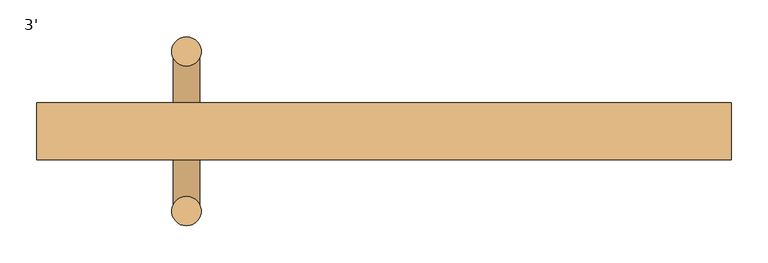
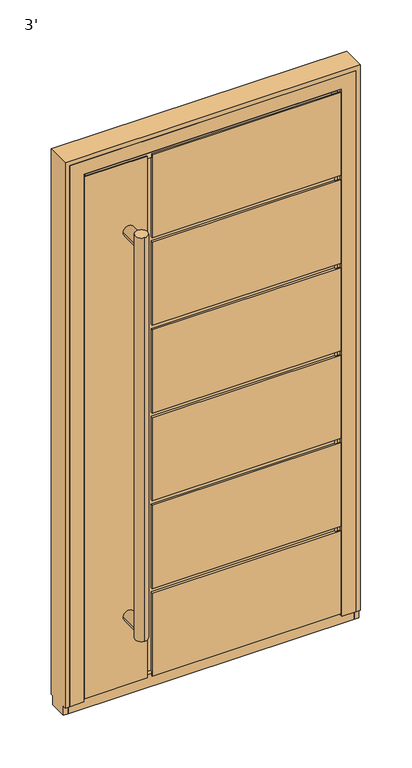
"""IFC4 building model written with IfcOpenShell, lengths in millimetres: door geometry, 3'."""

from ifc_helpers import new_model, si_unit, point, frame, frame_2d, origin, place, context, project, spatial, circle_curve, trimmed, segment, composite_curve, outline, extrude, faceted_brep, source, transform, mapped, element, save


def door_3_44036f4b(model_context):
    return source(origin(), model_context, "Body", "SolidModel", [
        extrude(outline(composite_curve([segment(trimmed(circle_curve(frame_2d((-268.65, 90.8003001)), 20.0), [point((-268.65, 70.8003001))], [point((-268.65, 110.8003001))], False, "CARTESIAN"), True, "CONTINUOUS"), segment(trimmed(circle_curve(frame_2d((-268.65, 90.8003001)), 20.0), [point((-268.65, 110.8003001))], [point((-268.65, 70.8003001))], False, "CARTESIAN"), True, "CONTINUOUS")], self_intersect=False)), frame((0.0, 0.0, 210.0000003), z_axis=(0.0, 0.0, 1.0), x_axis=(1.0, 0.0, 0.0)), (0.0, 0.0, 1.0), 1363.8),
        extrude(outline(composite_curve([segment(trimmed(circle_curve(frame_2d((-268.65, -126.2003001)), 20.0), [point((-268.65, -146.2003001))], [point((-268.65, -106.2003001))], False, "CARTESIAN"), True, "CONTINUOUS"), segment(trimmed(circle_curve(frame_2d((-268.65, -126.2003001)), 20.0), [point((-268.65, -106.2003001))], [point((-268.65, -146.2003001))], False, "CARTESIAN"), True, "CONTINUOUS")], self_intersect=False)), frame((0.0, 0.0, 210.0000003), z_axis=(0.0, 0.0, 1.0), x_axis=(1.0, 0.0, 0.0)), (0.0, 0.0, 1.0), 1363.8),
        extrude(outline(composite_curve([segment(trimmed(circle_curve(frame_2d((241.9000003, -268.65)), 18.0), [point((241.9000003, -286.65))], [point((241.9000003, -250.65))], False, "CARTESIAN"), True, "CONTINUOUS"), segment(trimmed(circle_curve(frame_2d((241.9000003, -268.65)), 18.0), [point((241.9000003, -250.65))], [point((241.9000003, -286.65))], False, "CARTESIAN"), True, "CONTINUOUS")], self_intersect=False)), frame((0.0, -126.2, 0.0), z_axis=(0.0, 1.0, 0.0), x_axis=(0.0, 0.0, 1.0)), (0.0, 0.0, 1.0), 217.0),
        extrude(outline(composite_curve([segment(trimmed(circle_curve(frame_2d((1541.9000003, -268.65)), 18.0), [point((1541.9000003, -286.65))], [point((1541.9000003, -250.65))], False, "CARTESIAN"), True, "CONTINUOUS"), segment(trimmed(circle_curve(frame_2d((1541.9000003, -268.65)), 18.0), [point((1541.9000003, -250.65))], [point((1541.9000003, -286.65))], False, "CARTESIAN"), True, "CONTINUOUS")], self_intersect=False)), frame((0.0, -126.2, 0.0), z_axis=(0.0, 1.0, 0.0), x_axis=(0.0, 0.0, 1.0)), (0.0, 0.0, 1.0), 217.0),
        faceted_brep([(-193.65, 13.8, 306.466667), (383.65, 13.8, 306.466667), (383.65, 13.8, 291.466667), (-193.65, 13.8, 291.466667), (-193.65, 13.8, 35.0), (-208.65, 13.8, 35.0), (-208.65, 13.8, 1748.8000003), (-193.65, 13.8, 1748.8000003), (-193.65, 13.8, 1492.3333337), (383.65, 13.8, 1492.3333337), (383.65, 13.8, 1477.3333337), (-193.65, 13.8, 1477.3333337), (-193.65, 13.8, 1195.866667), (383.65, 13.8, 1195.866667), (383.65, 13.8, 1180.866667), (-193.65, 13.8, 1180.866667), (-193.65, 13.8, 899.4000004), (383.65, 13.8, 899.4000004), (383.65, 13.8, 884.4000004), (-193.65, 13.8, 884.4000004), (-193.65, 13.8, 602.9333337), (383.65, 13.8, 602.9333337), (383.65, 13.8, 587.9333337), (-193.65, 13.8, 587.9333337), (-193.65, 20.8, 587.9333337), (-193.65, 20.8, 306.466667), (383.65, 20.8, 587.9333337), (383.65, 11.7997698, 1748.8000003), (383.65, 11.7997698, 35.0), (383.65, 18.8020472, 35.0), (383.65, 18.8020472, 24.0), (383.65, 20.8, 24.0), (383.65, 20.8, 291.466667), (383.65, 20.8, 306.466667), (383.65, 20.8, 602.9333337), (383.65, 20.8, 884.4000004), (383.65, 20.8, 899.4000004), (383.65, 20.8, 1180.866667), (383.65, 20.8, 1195.866667), (383.65, 20.8, 1477.3333337), (383.65, 20.8, 1492.3333337), (383.65, 20.8, 1748.8000003), (-193.65, 20.8, 602.9333337), (-193.65, 20.8, 884.4000004), (-193.65, 20.8, 899.4000004), (-193.65, 20.8, 1180.866667), (-208.65, 18.8020472, 35.0), (-208.65, 18.8020472, 24.0), (-208.65, 20.8, 24.0), (-208.65, 20.8, 1748.8000003), (-383.65, 11.7997698, 35.0), (-383.65, 18.8020472, 35.0), (-193.65, 18.8020472, 35.0), (-193.65, 20.8, 291.466667), (-193.65, 20.8, 24.0), (-193.65, 18.8020472, 24.0), (-383.65, 18.8020472, 24.0), (-383.65, 20.8, 24.0), (-383.65, 20.8, 1748.8000003), (-193.65, 20.8, 1195.866667), (-193.65, 20.8, 1477.3333337), (-193.65, 20.8, 1492.3333337), (-193.65, 20.8, 1748.8000003), (408.65, -56.2, 10.0000003), (-193.65, -56.2, 10.0000003), (-193.65, -53.2, 10.0000003), (408.65, -53.2, 10.0000003), (-408.65, -53.2, 10.0000003), (-208.65, -53.2, 10.0000003), (-208.65, -56.2, 10.0000003), (-408.65, -56.2, 10.0000003), (408.65, -56.2, 306.466667), (408.65, -53.2, 306.466667), (408.65, -53.2, 587.9333337), (408.65, -56.2, 587.9333337), (408.65, -56.2, 899.4000004), (408.65, -53.2, 899.4000004), (408.65, -53.2, 1180.866667), (408.65, -56.2, 1180.866667), (408.65, -56.2, 602.9333337), (408.65, -53.2, 602.9333337), (408.65, -53.2, 884.4000004), (408.65, -56.2, 884.4000004), (408.65, -56.2, 1195.866667), (408.65, -53.2, 1195.866667), (408.65, -53.2, 1477.3333337), (408.65, -56.2, 1477.3333337), (408.65, -56.2, 1773.8000003), (408.65, -56.2, 1492.3333337), (408.65, -53.2, 1492.3333337), (408.65, -53.2, 1773.8000003), (408.65, -53.2, 291.466667), (408.65, -56.2, 291.466667), (-193.65, -53.2, 25.5), (393.15, -53.2, 25.5), (393.15, -53.2, 291.466667), (393.15, -53.2, 306.466667), (393.15, -53.2, 587.9333337), (393.15, -53.2, 899.4000004), (393.15, -53.2, 1180.866667), (393.15, -53.2, 602.9333337), (393.15, -53.2, 884.4000004), (-393.15, -53.2, 25.5), (-208.65, -53.2, 25.5), (-408.65, -53.2, 1773.8000003), (-208.65, -53.2, 1773.8000003), (-208.65, -53.2, 1758.3000003), (-393.15, -53.2, 1758.3000003), (393.15, -53.2, 1195.866667), (393.15, -53.2, 1477.3333337), (393.15, -53.2, 1492.3333337), (393.15, -53.2, 1758.3000003), (-193.65, -53.2, 1758.3000003), (-193.65, -53.2, 1773.8000003), (-193.65, -49.2, 291.466667), (-193.65, -49.2, 25.5), (-193.65, -56.2, 291.466667), (-208.65, -56.2, 1773.8000003), (-408.65, -56.2, 1773.8000003), (-193.65, -56.2, 587.9333337), (-193.65, -56.2, 306.466667), (-193.65, -56.2, 1180.866667), (-193.65, -56.2, 899.4000004), (-193.65, -56.2, 884.4000004), (-193.65, -56.2, 602.9333337), (-193.65, -56.2, 1477.3333337), (-193.65, -56.2, 1195.866667), (-193.65, -56.2, 1773.8000003), (-193.65, -56.2, 1492.3333337), (-208.65, -49.2, 1758.3000003), (-208.65, -49.2, 25.5), (-383.65, 11.7997698, 1748.8000003), (393.15, 11.7997698, 1758.3000003), (393.15, 11.7997698, 25.5), (-393.15, 11.7997698, 25.5), (-393.15, 11.7997698, 1758.3000003), (393.15, -49.2, 1492.3333337), (393.15, -49.2, 1477.3333337), (393.15, -49.2, 1195.866667), (393.15, -49.2, 1180.866667), (393.15, -49.2, 899.4000004), (393.15, -49.2, 884.4000004), (393.15, -49.2, 602.9333337), (393.15, -49.2, 587.9333337), (393.15, -49.2, 306.466667), (393.15, -49.2, 291.466667), (-193.65, -49.2, 1477.3333337), (-193.65, -49.2, 1492.3333337), (-193.65, -49.2, 1758.3000003), (-193.65, -49.2, 306.466667), (-193.65, -49.2, 587.9333337), (-193.65, -49.2, 602.9333337), (-193.65, -49.2, 884.4000004), (-193.65, -49.2, 899.4000004), (-193.65, -49.2, 1180.866667), (-193.65, -49.2, 1195.866667)], [[[0, 1, 2, 3, 4, 5, 6, 7, 8, 9, 10, 11, 12, 13, 14, 15, 16, 17, 18, 19, 20, 21, 22, 23]], [[23, 24, 25, 0]], [[23, 22, 26, 24]], [[27, 28, 29, 30, 31, 32, 2, 1, 33, 26, 22, 21, 34, 35, 18, 17, 36, 37, 14, 13, 38, 39, 10, 9, 40, 41]], [[42, 34, 21, 20]], [[19, 43, 42, 20]], [[19, 18, 35, 43]], [[44, 36, 17, 16]], [[15, 45, 44, 16]], [[5, 46, 47, 48, 49, 6]], [[28, 50, 51, 46, 5, 4, 52, 29]], [[53, 54, 55, 52, 4, 3]], [[3, 2, 32, 53]], [[25, 33, 1, 0]], [[29, 52, 55, 30]], [[56, 47, 46, 51]], [[30, 55, 54, 31]], [[57, 48, 47, 56]], [[36, 44, 45, 37]], [[34, 42, 43, 35]], [[33, 25, 24, 26]], [[54, 53, 32, 31]], [[58, 49, 48, 57]], [[38, 59, 60, 39]], [[41, 40, 61, 62]], [[63, 64, 65, 66]], [[67, 68, 69, 70]], [[71, 72, 73, 74]], [[75, 76, 77, 78]], [[79, 80, 81, 82]], [[83, 84, 85, 86]], [[87, 88, 89, 90]], [[66, 91, 92, 63]], [[65, 93, 94, 95, 91, 66]], [[72, 96, 97, 73]], [[76, 98, 99, 77]], [[80, 100, 101, 81]], [[102, 103, 68, 67, 104, 105, 106, 107]], [[84, 108, 109, 85]], [[90, 89, 110, 111, 112, 113]], [[114, 115, 93, 65, 64, 116]], [[70, 69, 117, 118]], [[63, 92, 116, 64]], [[74, 119, 120, 71]], [[78, 121, 122, 75]], [[82, 123, 124, 79]], [[86, 125, 126, 83]], [[87, 127, 128, 88]], [[70, 118, 104, 67]], [[129, 106, 105, 117, 69, 68, 103, 130]], [[58, 57, 56, 51, 50, 131]], [[132, 133, 134, 135], [131, 50, 28, 27]], [[111, 110, 136, 137, 109, 108, 138, 139, 99, 98, 140, 141, 101, 100, 142, 143, 97, 96, 144, 145, 95, 94, 133, 132]], [[94, 93, 115, 130, 103, 102, 134, 133]], [[135, 134, 102, 107]], [[146, 137, 136, 147, 148, 129, 130, 115, 114, 145, 144, 149, 150, 143, 142, 151, 152, 141, 140, 153, 154, 139, 138, 155]], [[153, 122, 121, 154]], [[153, 140, 98, 76, 75, 122]], [[123, 82, 81, 101, 141, 152]], [[151, 124, 123, 152]], [[151, 142, 100, 80, 79, 124]], [[119, 74, 73, 97, 143, 150]], [[149, 120, 119, 150]], [[149, 144, 96, 72, 71, 120]], [[116, 92, 91, 95, 145, 114]], [[15, 14, 37, 45]], [[59, 38, 13, 12]], [[11, 60, 59, 12]], [[11, 10, 39, 60]], [[61, 40, 9, 8]], [[8, 7, 62, 61]], [[125, 86, 85, 109, 137, 146]], [[128, 127, 113, 112, 148, 147]], [[121, 78, 77, 99, 139, 154]], [[155, 138, 108, 84, 83, 126]], [[155, 126, 125, 146]], [[147, 136, 110, 89, 88, 128]], [[90, 113, 127, 87]], [[118, 117, 105, 104]], [[132, 135, 107, 106, 129, 148, 112, 111]], [[27, 41, 62, 7, 6, 49, 58, 131]]]),
        faceted_brep([(-457.2, -56.2, 0.0), (-457.2, -47.1997571, 0.0), (-412.7, -47.1997571, 0.0), (-412.7, -56.2, 0.0), (-403.2, 16.2999958, 0.0), (-403.2, 11.8, 0.0), (-457.2, 11.8, 0.0), (-457.2, 20.8, 0.0), (-387.7, 20.8, 0.0), (-387.7, 16.2999958, 0.0), (457.2, 20.8, 0.0), (457.2, 11.8, 0.0), (403.2, 11.8, 0.0), (403.2, 16.2999958, 0.0), (387.7, 16.2999958, 0.0), (387.7, 20.8, 0.0), (412.7, -47.1997571, 0.0), (457.2, -47.1997571, 0.0), (457.2, -56.2, 0.0), (412.7, -56.2, 0.0), (-457.2, 11.8, -30.0), (-457.2, -47.1997571, -30.0), (-457.2, -56.2, 1828.8), (-457.2, 20.8, 1828.8), (-412.7, -56.2, 1784.3), (412.7, -56.2, 1784.3), (457.2, -56.2, 1828.8), (457.2, 20.8, 1828.8), (457.2, -47.1997571, -30.0), (457.2, 11.8, -30.0), (387.7, 20.8, 1759.3), (-387.7, 20.8, 1759.3), (-403.2, -47.2, 1774.8), (-403.2, -47.2, 14.5), (-403.2, 11.8, 14.5), (-403.2, 16.2999958, 1774.8), (403.2, 16.2999958, 1774.8), (403.2, -47.2, 1774.8), (403.2, 11.8, 14.5), (403.2, -47.2, 14.5), (-412.7, -47.2, 1784.3), (412.7, -47.2, 1784.3), (-387.7, 16.2999958, 1759.3), (387.7, 16.2999958, 1759.3)], [[[0, 1, 2, 3]], [[4, 5, 6, 7, 8, 9]], [[10, 11, 12, 13, 14, 15]], [[16, 17, 18, 19]], [[7, 6, 20, 21, 1, 0, 22, 23]], [[3, 24, 25, 19, 18, 26, 22, 0]], [[22, 26, 27, 23]], [[18, 17, 28, 29, 11, 10, 27, 26]], [[7, 23, 27, 10, 15, 30, 31, 8]], [[32, 33, 34, 5, 4, 35]], [[35, 36, 37, 32]], [[36, 13, 12, 38, 39, 37]], [[40, 24, 3, 2]], [[16, 41, 40, 2, 1, 21, 28, 17], [37, 39, 33, 32]], [[9, 42, 43, 14, 13, 36, 35, 4]], [[8, 31, 42, 9]], [[24, 40, 41, 25]], [[30, 43, 42, 31]], [[19, 25, 41, 16]], [[14, 43, 30, 15]], [[20, 6, 5, 34, 38, 12, 11, 29]], [[39, 38, 34, 33]], [[20, 29, 28, 21]]]),
        faceted_brep([(-457.2, -47.2, -30.0), (-472.2, -47.2, -30.0), (-472.2, 11.8, -30.0), (-457.2, 11.8, -30.0), (-457.2, -56.2, 1828.8), (-457.2, -56.2, 0.0), (-457.2, -47.2, 0.0), (-457.2, 11.8, 0.0), (-457.2, 20.8, 0.0), (-457.2, 20.8, 1828.8), (-472.2, 11.8, 0.0), (472.2, 11.8, 0.0), (472.2, 11.8, -30.0), (457.2, 11.8, -30.0), (457.2, 11.8, 0.0), (-472.2, 20.8, 1843.8), (-472.2, 20.8, 0.0), (-472.2, -47.2, 0.0), (-472.2, -56.2, 0.0), (-472.2, -56.2, 1843.8), (457.2, -47.2, 0.0), (457.2, -47.2, -30.0), (472.2, -47.2, -30.0), (472.2, -47.2, 0.0), (457.2, 20.8, 1828.8), (457.2, 20.8, 0.0), (457.2, -56.2, 0.0), (457.2, -56.2, 1828.8), (472.2, -56.2, 0.0), (472.2, -56.2, 1843.8), (472.2, 20.8, 0.0), (472.2, 20.8, 1843.8)], [[[0, 1, 2, 3]], [[4, 5, 6, 0, 3, 7, 8, 9]], [[7, 3, 2, 10]], [[11, 12, 13, 14]], [[15, 16, 10, 2, 1, 17, 18, 19]], [[17, 1, 0, 6]], [[20, 21, 22, 23]], [[24, 25, 14, 13, 21, 20, 26, 27]], [[27, 26, 28, 29, 19, 18, 5, 4]], [[6, 5, 18, 17]], [[23, 28, 26, 20]], [[22, 21, 13, 12]], [[10, 16, 8, 7]], [[14, 25, 30, 11]], [[9, 8, 16, 15, 31, 30, 25, 24]], [[29, 28, 23, 22, 12, 11, 30, 31]], [[9, 24, 27, 4]], [[19, 29, 31, 15]]]),
    ])


if __name__ == "__main__":
    model = new_model("IFC4")
    model_context = context("Model", 3, world=origin())
    ifc_project = project(units=[si_unit("LENGTHUNIT", "METRE", prefix="MILLI")], contexts=[model_context])
    site = spatial("IfcSite", under=ifc_project)
    building = spatial("IfcBuilding", under=site)
    placement = place(None, origin())
    door_3_shape = door_3_44036f4b(model_context)
    element("IfcDoor", 1, ObjectType="3'", at=placement, inside=building, context=model_context, shape_type="MappedRepresentation", body=[
        mapped(door_3_shape, transform((0.0, 0.0, 0.0), x_axis=(1.0, 0.0, 0.0), y_axis=(0.0, 1.0, 0.0), z_axis=(0.0, 0.0, 1.0))),
    ])
    save(model, "model.ifc")

# Revit data of these elements
# Type "3'"
#   Type Mark = "9"
#   Water resistance = "up to Class E900, EN 12208:2001"
#   Uniclass2015Version = "v1.21"
#   Uniclass2015Reference = "Ss_25_30_20_30"
#   Uniclass2015Description = "Frame and door leaf system"
#   URL = "www.aluprof.com"
#   Type IFC Predefined Type = "USERDEFINED"
#   Right-hand / Left-hand door [instance default] = ""
#   Resistance to wind load = "up to Class C5/B5, EN 12210:2001"
#   Insert type = "ST"
#   Hardware [instance default] = ""
#   Product page = "https://aluprof.com/en/architects/offer/window-and-door-systems/panel-doors#visualisation"
#   Operation = "SinglePanelOutwardOpening"
#   Opening type = "Outward"
#   NBSReference = "25-50-20/125"
#   NBSDescription = "Frame and door leaf system"
#   Important = "The actual acceptable construction dimensions are dependent on the selection of profiles and hardware, glazing type, construction weight and the construction’s operating conditions. These should be determined by a suitably qualified person, and using ALUPROF’s calculation software"
#   IfcExportType = "USERDEFINED"
#   IfcExportAs = "IfcDoorType"
#   Handle type [instance default] = ""
#   Manufacturer = "ALUPROF SA"
#   Export Type to IFC As = "IfcDoorType"
#   Door sill type [instance default] = ""
#   Description = "External single-leaf panel door outward opening"
#   Model = "MB-86 ST Panel Door AD07"
#   Content of the recyclate in the material = "69.2%"
#   COBie.Type.WarrantyDurationParts = ""
#   COBie.Type.Name = ""
#   COBie.Type.Manufacturer = "ALUPROF SA"
#   COBie.Space.Name = ""
#   COBie.Floor.Name = ""
#   COBie.Facility.Name = ""
#   COBie.CreatedOn = ""
#   COBie.Component.WarrantyStartDate = ""
#   COBie.Component.Name = "MB-86 ST Panel Door AD07"
#   Burglar resistance = "RC2"
#   Air permeability = "up to Class 4, EN 12207:2001"
#   Width of the active leaf = 2' - 8.17717"
#   Placement in wall = 0' - 0.7874"
#   Thickness = 0' - 3.0315"
#   Height of the opening sash = 5' - 9.44094"
#   Handle Offset = 3' - 5.33858"
#   Rough Height = 6' - 2.40945"
#   Rough Width = 3' - 1.1811"
#   Height = 6' - 0"
#   Width = 3' - 0"
#   Construction depth = 0' - 3.0315"
#   Clear opening width = 2' - 3.94882"
#   Clear opening height = 5' - 8.47638"
#   Height of the array = 0' - 11.08136"
#   Schedule No. [instance default] = 1
#   Handrail [instance default] = yes
#   IsExternal = yes
#   Handle [instance default] = no
#   Door closer [instance default] = no
#   Function = 1
#   COBie.Type = yes
#   COBie = yes
#   Access control [instance default] = no
#   Panel = element 380416
#   Wall Closure = (empty or 0)
